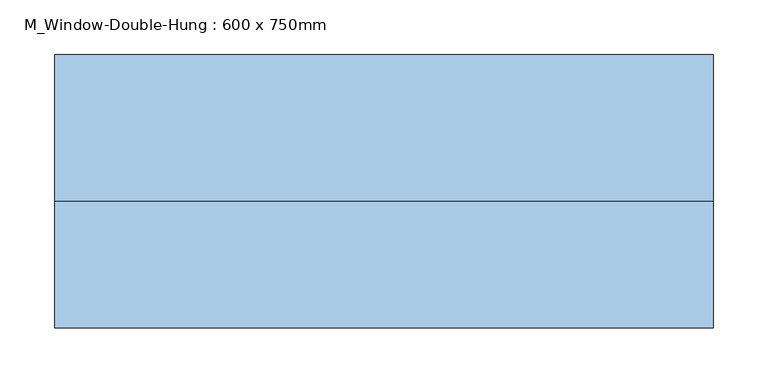
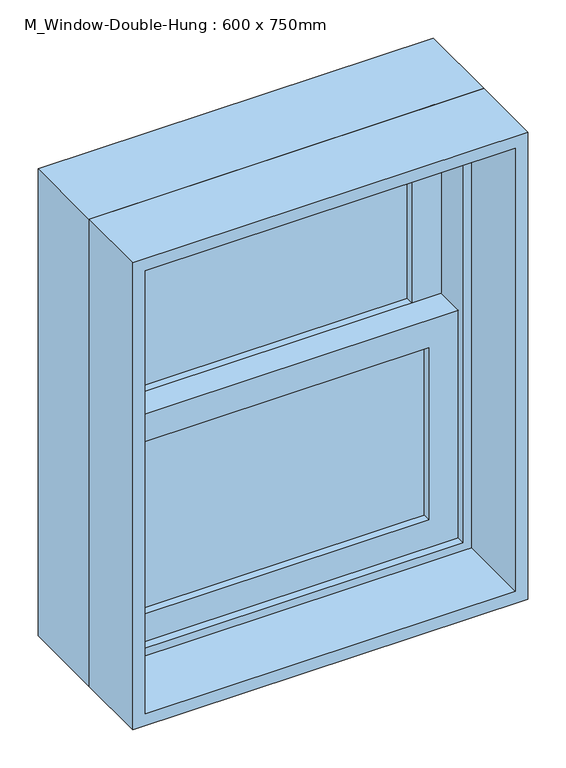
"""IFC4 building model written with IfcOpenShell, lengths in millimetres: window geometry, M_Window-Double-Hung : 600 x 750mm."""

from ifc_helpers import new_model, si_unit, frame, origin, place, context, project, spatial, polyline, outline, extrude, source, transform, mapped, element, save


def m_window_double_hung_600_x_750mm_49d140ec(model_context):
    return source(origin(), model_context, "Body", "SweptSolid", [
        extrude(outline(polyline([(223.8, 45.15), (223.8, 38.8), (-223.8, 38.8), (-223.8, 45.15), (223.8, 45.15)])), frame((0.0, 0.0, 990.6), z_axis=(0.0, 0.0, 1.0), x_axis=(1.0, 0.0, 0.0)), (0.0, 0.0, 1.0), 276.575),
        extrude(outline(polyline([(-223.8, 32.45), (223.8, 32.45), (223.8, 26.1), (-223.8, 26.1), (-223.8, 32.45)])), frame((0.0, 0.0, 990.6), z_axis=(0.0, 0.0, 1.0), x_axis=(1.0, 0.0, 0.0)), (0.0, 0.0, 1.0), 276.575),
        extrude(outline(polyline([(223.8, 89.6), (223.8, 83.25), (-223.8, 83.25), (-223.8, 89.6), (223.8, 89.6)])), frame((0.0, 0.0, 1311.625), z_axis=(0.0, 0.0, 1.0), x_axis=(1.0, 0.0, 0.0)), (0.0, 0.0, 1.0), 276.575),
        extrude(outline(polyline([(-223.8, 76.9), (223.8, 76.9), (223.8, 70.55), (-223.8, 70.55), (-223.8, 76.9)])), frame((0.0, 0.0, 1311.625), z_axis=(0.0, 0.0, 1.0), x_axis=(1.0, 0.0, 0.0)), (0.0, 0.0, 1.0), 276.575),
        extrude(outline(polyline([(1311.625, -268.25), (946.15, -268.25), (946.15, 268.25), (1311.625, 268.25), (1311.625, -268.25)]), holes=[polyline([(1267.175, 223.8), (990.6, 223.8), (990.6, -223.8), (1267.175, -223.8), (1267.175, 223.8)])]), frame((0.0, 13.4, 0.0), z_axis=(0.0, 1.0, 0.0), x_axis=(0.0, 0.0, 1.0)), (0.0, 0.0, 1.0), 44.45),
        extrude(outline(polyline([(1632.65, -268.25), (1267.175, -268.25), (1267.175, 268.25), (1632.65, 268.25), (1632.65, -268.25)]), holes=[polyline([(1588.2, 223.8), (1311.625, 223.8), (1311.625, -223.8), (1588.2, -223.8), (1588.2, 223.8)])]), frame((0.0, 57.85, 0.0), z_axis=(0.0, 1.0, 0.0), x_axis=(0.0, 0.0, 1.0)), (0.0, 0.0, 1.0), 44.45),
        extrude(outline(polyline([(1664.4, -300.0), (914.4, -300.0), (914.4, 300.0), (1664.4, 300.0), (1664.4, -300.0)]), holes=[polyline([(1632.65, 268.25), (946.15, 268.25), (946.15, -268.25), (1632.65, -268.25), (1632.65, 268.25)])]), frame((0.0, 0.7, 0.0), z_axis=(0.0, 1.0, 0.0), x_axis=(0.0, 0.0, 1.0)), (0.0, 0.0, 1.0), 133.35),
        extrude(outline(polyline([(1664.4, 300.0), (1664.4, -300.0), (914.4, -300.0), (914.4, 300.0), (1664.4, 300.0)]), holes=[polyline([(1645.35, 280.95), (933.45, 280.95), (933.45, -280.95), (1645.35, -280.95), (1645.35, 280.95)])]), frame((0.0, -115.0, 0.0), z_axis=(0.0, 1.0, 0.0), x_axis=(0.0, 0.0, 1.0)), (0.0, 0.0, 1.0), 115.7),
    ])


if __name__ == "__main__":
    model = new_model("IFC4")
    model_context = context("Model", 3, world=origin())
    ifc_project = project(units=[si_unit("LENGTHUNIT", "METRE", prefix="MILLI")], contexts=[model_context])
    site = spatial("IfcSite", under=ifc_project)
    building = spatial("IfcBuilding", under=site)
    placement = place(None, origin())
    m_window_double_hung_600_x_750mm_shape = m_window_double_hung_600_x_750mm_49d140ec(model_context)
    element("IfcWindow", 1, ObjectType="M_Window-Double-Hung : 600 x 750mm", at=placement, inside=building, context=model_context, shape_type="MappedRepresentation", body=[
        mapped(m_window_double_hung_600_x_750mm_shape, transform((0.0, 0.0, 0.0), x_axis=(1.0, 0.0, 0.0), y_axis=(0.0, 1.0, 0.0), z_axis=(0.0, 0.0, 1.0))),
    ])
    save(model, "model.ifc")

# Revit data of these elements
# Type "M_Window-Double-Hung : 600 x 750mm"
#   Type Mark = "V"
#   Fire Rating = "0.5h"
#   Construction Type Id = "DG-DR"
#   Assembly Code = "B2020100"
#   Analytic Construction = "Double glazing - domestic"
#   Wall Thickness [instance default] = 0.15 m
#   Window Inset [instance default] = 0 m
#   Visual Light Transmittance = 0.81
#   Thermal Resistance (R) = 0.319569 (m²·K)/W
#   Solar Heat Gain Coefficient = 0.76
#   Muntin Width = 0.4476 m
#   Muntin Height = 0.276575 m
#   Interior Wall Closure [instance default] = 0.0357 m
#   Rough Width = 0.615 m
#   Rough Height = 0.765 m
#   Frame Extension [instance default] = 0.03175 m
#   Exterior Wall Closure [instance default] = 0.0127 m
#   Extension Jamb [instance default] = 0.0357 m
#   Heat Transfer Coefficient (U) = 3.12929 W/(m²·K)
#   Height = 0.75 m
#   Width = 0.6 m
#   Top Muntin Visibility = yes
#   Indicator Visibility [instance default] = yes
#   Extension Jamb Visibility [instance default] = yes
#   Interior Trim Visibility [instance default] = yes
#   Exterior Trim Visibility [instance default] = yes
#   Define Thermal Properties by = 1
#   Bottom Muntin Visibility = yes
#   Muntin Pattern = M_Muntin Pattern_2x2 : M_Muntin Pattern_2x2
#   Interior Trim Material = Wood - Stained
#   Interior Trim = M_Trim-Window-Interior-Flat : Picture Frame
#   Exterior Trim Material = Clad - White
#   Exterior Trim = M_Trim-Window-Exterior-Flat : with Sill
#   Glass Panel Material = Glass
#   Exterior Frame Material = Clad - White
#   Interior Frame Material = Wood - Stained
#   Wall Closure = (empty or 0)
# Element 1 (IfcWindow, "M_Window-Double-Hung : 600 x 750mm")
#   Wall Thickness = 0.23 m
#   Extension Jamb = 0.1157 m
#   Materials on its faces: "Wood - Stained", "Glass", "Clad - White"
# Materials
#   "Wood - Stained": class "Wood", colour RGB 224 178 126, transparency 0, Cost = 0
#   "Clad - White": class "Wood", colour RGB 242 242 238, transparency 0, Cost = 0
#   "Glass": class "Glass", colour RGB 0 128 192, transparency 0.9, Description = "Soda Lime Glass", Cost = 0
